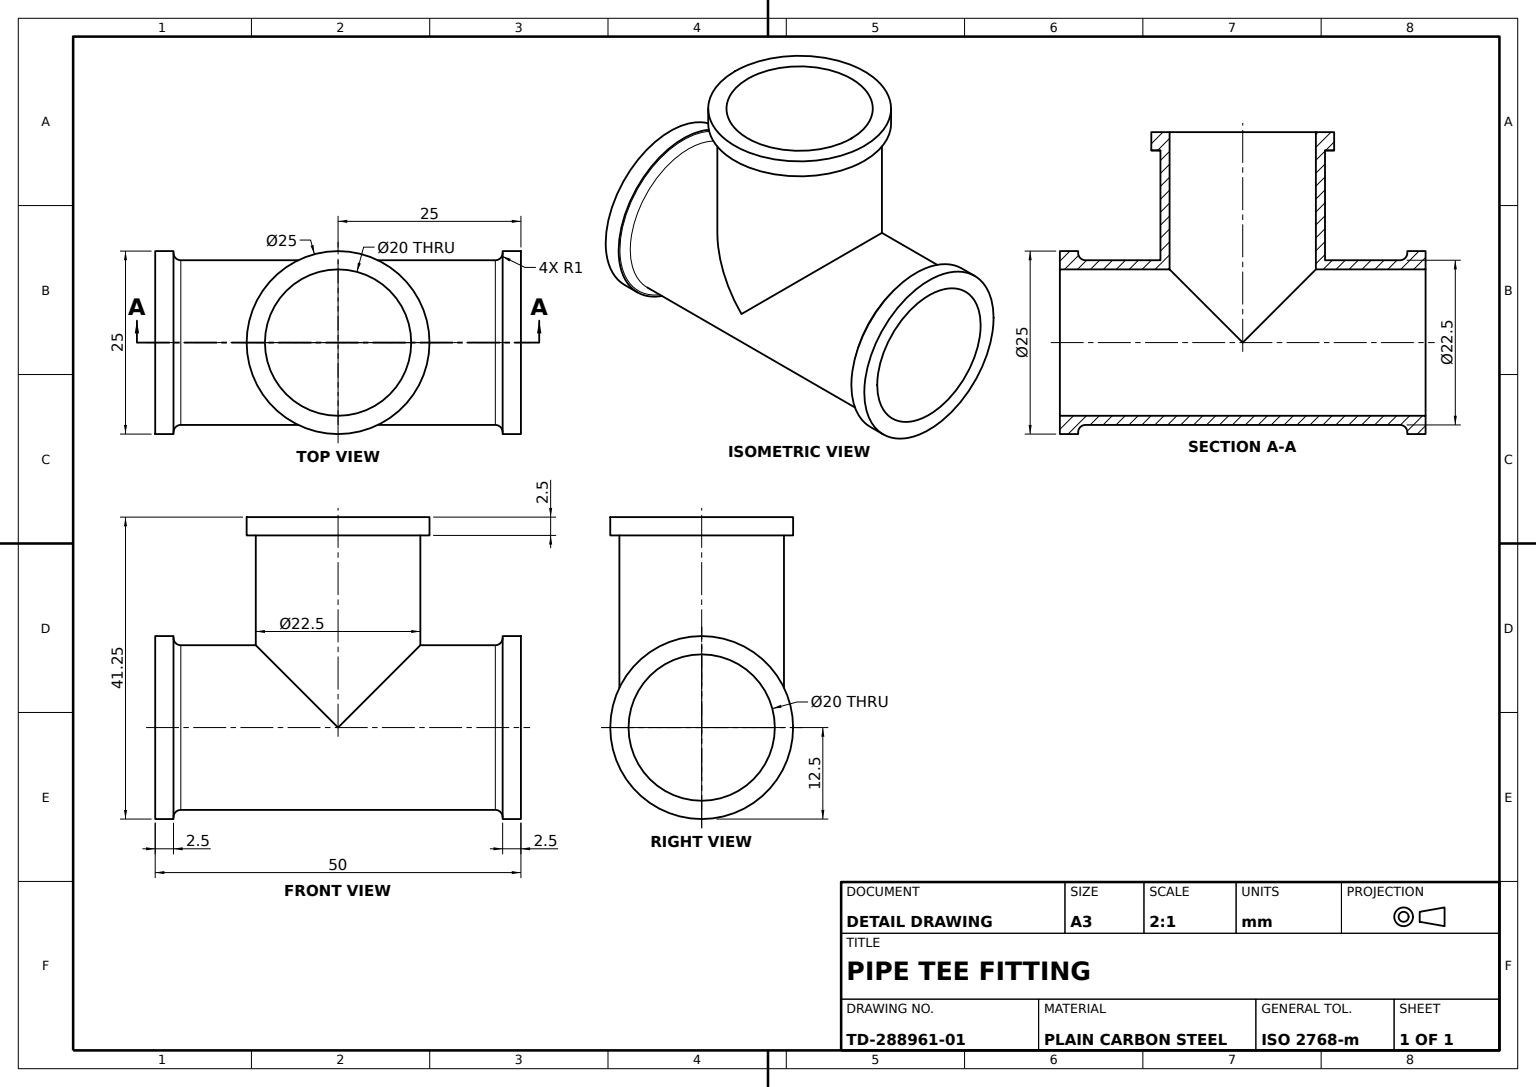
SolidWorks part; units mm, degrees
material "Plain Carbon Steel"
ref_plane "Front Plane" through (0, 0, 0) normal (0, 0, 1) x (1, 0, 0)
ref_plane "Top Plane" through (0, 0, 0) normal (0, 1, 0) x (1, 0, 0)
ref_plane "Right Plane" through (0, 0, 0) normal (1, 0, 0) x (0, 0, -1)
sketch "End Rim A Profile Ø25" plane through (0, 0, 0) normal (0, 0, 1) x (1, 0, 0)
  circle A0 centre (0, 0) radius 12.5
  dimension "D1" = 25
extrude "End Rim A Ø25" add sketch "End Rim A Profile Ø25" along normal mid plane 2.5
sketch "Run Tube Profile Ø22.5" plane through (0, 0, 1.25) normal (0, 0, 1) x (1, 0, 0)
  circle A0 centre (0, 0) radius 11.25
  dimension "D1" = 22.5
extrude "Run Tube Ø22.5" add sketch "Run Tube Profile Ø22.5" against normal blind 45 from offset 2.5 offset against normal yes
ref_plane "Plane1" through (0, 0, -22.5) normal (0, 0, 1) x (1, 0, 0)
sketch "End Rim B Profile Ø25" plane through (0, 0, -46.25) normal (0, 0, -1) x (-1, 0, 0)
  circle A0 centre (0, 0) radius 12.5
  dimension "D1" = 25
extrude "End Rim B Ø25" add sketch "End Rim B Profile Ø25" along normal blind 2.5
sketch "Run Bore Profile Ø20" plane through (0, 0, -48.75) normal (0, 0, -1) x (-1, 0, 0)
  circle A0 centre (0, 0) radius 10
  dimension "D1" = 20
extrude "Run Bore Ø20" cut sketch "Run Bore Profile Ø20" against normal through all
fillet "Rim Fillets R1" radius 1 2 edges at (11.25, 0, -1.25) (11.25, 0, -46.25)
sketch "Branch Rim Profile Ø25" plane through (0, 0, 0) normal (0, 1, 0) x (1, 0, 0)
  line L0 (0, 48.75) -> (0, -1.25)
  line L1 (10, 48.75) -> (-10, 48.75) construction
  line L2 (-12.5, -1.25) -> (12.5, -1.25) construction
  circle A0 centre (0, 23.75) radius 12.5
  dimension "D1" = 25
extrude "Branch Rim Ø25" add sketch "Branch Rim Profile Ø25" along normal blind 2.5 from offset 26.25 separate body contours L0 A0 | L0 A0
sketch "Branch Tube Profile Ø22.5" plane through (0, 0, 0) normal (0, 1, 0) x (1, 0, 0)
  circle A2 centre (0, 23.75) radius 11.25
  dimension "D1" = 23.75
  dimension "D2" = 22.5
extrude "Branch Tube Ø22.5" add sketch "Branch Tube Profile Ø22.5" along normal blind 27
sketch "Run Bore Clearance Profile" plane through (0, 0, 1.25) normal (0, 0, 1) x (1, 0, 0)
  circle A0 centre (0, 0) radius 10
  dimension "D1" = 20
extrude "Run Bore Clearance Cut" cut sketch "Run Bore Clearance Profile" against normal through all
sketch "Branch Bore Profile Ø20" plane through (0, 28.75, 0) normal (0, 1, 0) x (1, 0, 0)
  circle A0 centre (0, 23.75) radius 10
  dimension "D1" = 20
extrude "Branch Bore Ø20" cut sketch "Branch Bore Profile Ø20" against normal up to next
